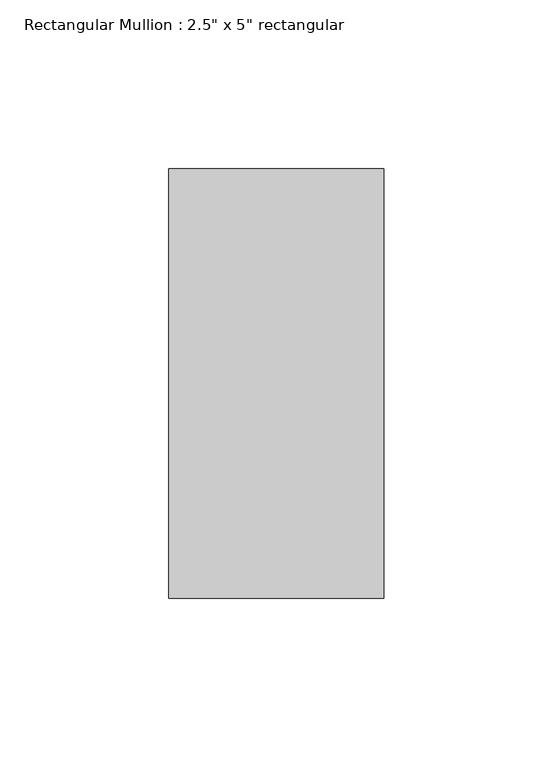
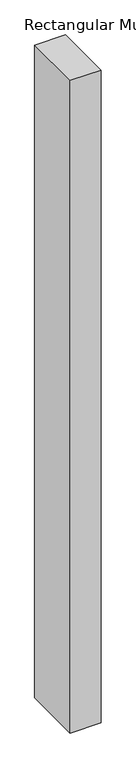
"""IFC4 building model written with IfcOpenShell, lengths in millimetres: member geometry."""

from ifc_helpers import new_model, si_unit, frame, origin, place, context, project, spatial, polyline, outline, extrude, source, transform, mapped, element, save


def member_2e151cea(model_context):
    return source(origin(), model_context, "Body", "SweptSolid", [
        extrude(outline(polyline([(0.0, 63.5), (0.0, -63.5), (-63.5, -63.5), (-63.5, 63.5), (0.0, 63.5)])), frame((0.0, 0.0, -1426.6333333), z_axis=(0.0, 0.0, 1.0), x_axis=(1.0, 0.0, 0.0)), (0.0, 0.0, 1.0), 1426.6333333),
    ])


if __name__ == "__main__":
    model = new_model("IFC4")
    model_context = context("Model", 3, world=origin())
    ifc_project = project(units=[si_unit("LENGTHUNIT", "METRE", prefix="MILLI")], contexts=[model_context])
    site = spatial("IfcSite", under=ifc_project)
    building = spatial("IfcBuilding", under=site)
    placement = place(None, origin())
    member_shape = member_2e151cea(model_context)
    element("IfcMember", 1, ObjectType="Rectangular Mullion : 2.5\" x 5\" rectangular", at=placement, inside=building, context=model_context, shape_type="MappedRepresentation", body=[
        mapped(member_shape, transform((0.0, 0.0, 0.0), x_axis=(1.0, 0.0, 0.0), y_axis=(0.0, 1.0, 0.0), z_axis=(0.0, 0.0, 1.0))),
    ])
    save(model, "model.ifc")

# Revit data of these elements
# Type "Rectangular Mullion : 2.5\" x 5\" rectangular"
#   built-in parameter 1007304 = 0.416667 (stored number, unit not read)
#   built-in parameter 1007301 = 0.104167 (stored number, unit not read)
#   built-in parameter 1007300 = 0.104167 (stored number, unit not read)
# Element 1 (IfcMember, "Rectangular Mullion : 2.5\" x 5\" rectangular")
#   Materials on its faces: "Aluminum"
# Materials
#   "Aluminum": class "Metal", colour RGB 247 247 247, transparency 0, Description = "Aluminum 6061", Cost = 0
